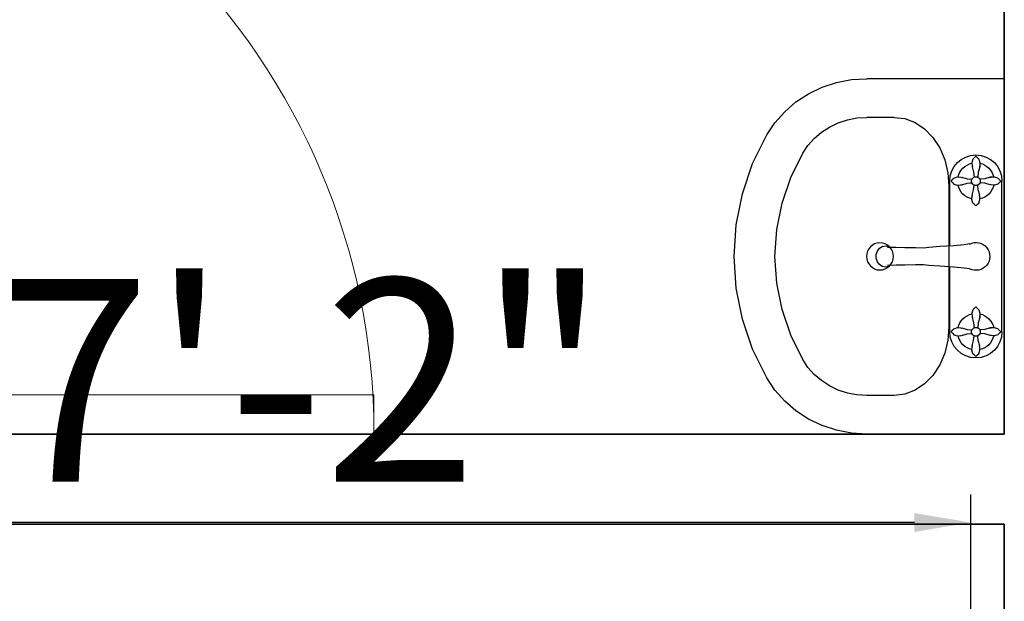
# Model space of a CAD drawing. Units: inches. Extents: x 3321 to 5237, y 11 to 1752.
# Tile 19 of 43: x 4413 to 4456, y 1280 to 1306. Entities that reach past the tile are written whole.
import ezdxf

# ---------------------------------------------------------------- set-up
doc = ezdxf.new("R2010")
doc.units = ezdxf.units.IN
for name, color, linetype, lineweight in [('A-ANNO-DIMS', 2, 'Continuous', 18), ('A-DOOR', 4, 'Continuous', 18), ('A-WALL', 7, 'Continuous', 35), ('Сантехника', 7, 'Continuous', 18)]:
    doc.layers.add(name, color=color, linetype=linetype, lineweight=lineweight)
doc.layers.add('SANTEH', color=7, linetype='Continuous')
doc.styles.get("Standard").update_dxf_attribs({"font": 'arial.ttf'})
doc.dimstyles.new('ISO-25', dxfattribs={"dimtxt": 9, "dimasz": 2.5, "dimexe": 1.25, "dimexo": 0.625, "dimtad": 1, "dimdec": 1, "dimlunit": 3, "dimtxsty": 'Standard', "dimcen": 2.5, "dimclrd": 4, "dimclre": 4, "dimclrt": 256, "dimadec": 0, "dimazin": 0, "dimtfac": 1, "dimtdec": 1, "dimtmove": 0, "dimatfit": 3, "dimfxl": 1, "dimarcsym": 0})

# ---------------------------------------------------------------- blocks, each defined once
blk = doc.blocks.new('*U5')
for p, q in [((0, 0), (0, -6)), ((-30, 0), (-30, -6))]:
    blk.add_line(p, q)
blk.add_lwpolyline([(0, 0), (0, 30), (-1.75, 30), (-1.75, 0)], close=True)
blk.add_arc((0, 0), 30, 90, 180)
blk = doc.blocks.new('Basin 01_71')
at = {"layer": 'SANTEH'}
for p, q in [((0, 350), (0, 171.8)), ((460, 350), (0, 350)), ((132.5, 345.3), (130.2, 343.2)), ((132.5, 345.3), (130.2, 343.2)), ((132.5, 345.3), (130.2, 343.2)), ((132.5, 345.3), (130.2, 343.2)), ((132.5, 345.3), (130.2, 343.2)), ((132.5, 345.3), (130.2, 343.2)), ((132.5, 346.9), (327.5, 346.9)), ((132.5, 345.3), (134.7, 343.2)), ((132.5, 345.3), (134.7, 343.2)), ((132.5, 345.3), (134.7, 343.2)), ((132.5, 345.3), (134.7, 343.2)), ((132.5, 345.3), (134.7, 343.2)), ((132.5, 345.3), (134.7, 343.2)), ((327.5, 345.3), (325.2, 343.2)), ((327.5, 345.3), (325.2, 343.2)), ((327.5, 345.3), (325.2, 343.2)), ((327.5, 345.3), (325.2, 343.2)), ((327.5, 345.3), (325.2, 343.2)), ((327.5, 345.3), (325.2, 343.2)), ((327.5, 345.3), (329.7, 343.2)), ((327.5, 345.3), (329.7, 343.2)), ((327.5, 345.3), (329.7, 343.2)), ((327.5, 345.3), (329.7, 343.2)), ((327.5, 345.3), (329.7, 343.2)), ((327.5, 345.3), (329.7, 343.2)), ((460, 350), (460, 171.8)), ((128.5, 341.7), (127.2, 337.2)), ((128.5, 341.7), (127.2, 337.2)), ((128.5, 341.7), (127.2, 337.2)), ((128.5, 341.7), (127.2, 337.2)), ((128.5, 341.7), (127.2, 337.2)), ((128.5, 341.7), (127.2, 337.2)), ((127.2, 337.2), (127.5, 332.3)), ((127.2, 337.2), (127.5, 332.3)), ((127.2, 337.2), (127.5, 332.3)), ((127.2, 337.2), (127.5, 332.3)), ((127.2, 337.2), (127.5, 332.3)), ((127.2, 337.2), (127.5, 332.3)), ((127.5, 332.3), (128.4, 332)), ((127.5, 332.3), (128.4, 332)), ((127.5, 332.3), (128.4, 332)), ((127.5, 332.3), (128.4, 332)), ((127.5, 332.3), (128.4, 332)), ((127.5, 332.3), (128.4, 332)), ((128.4, 332), (127.6, 331.5)), ((128.4, 332), (127.6, 331.5)), ((128.4, 332), (127.6, 331.5)), ((128.4, 332), (127.6, 331.5)), ((128.4, 332), (127.6, 331.5)), ((128.4, 332), (127.6, 331.5)), ((130.2, 343.2), (128.5, 341.7)), ((130.2, 343.2), (128.5, 341.7)), ((130.2, 343.2), (128.5, 341.7)), ((130.2, 343.2), (128.5, 341.7)), ((130.2, 343.2), (128.5, 341.7)), ((130.2, 343.2), (128.5, 341.7)), ((134.7, 343.2), (136.4, 341.7)), ((134.7, 343.2), (136.4, 341.7)), ((134.7, 343.2), (136.4, 341.7)), ((134.7, 343.2), (136.4, 341.7)), ((134.7, 343.2), (136.4, 341.7)), ((134.7, 343.2), (136.4, 341.7)), ((136.4, 341.7), (137.7, 337.2)), ((136.4, 341.7), (137.7, 337.2)), ((136.4, 341.7), (137.7, 337.2)), ((136.4, 341.7), (137.7, 337.2)), ((136.4, 341.7), (137.7, 337.2)), ((136.4, 341.7), (137.7, 337.2)), ((137.4, 332.3), (136.6, 332)), ((137.4, 332.3), (136.6, 332)), ((137.4, 332.3), (136.6, 332)), ((137.4, 332.3), (136.6, 332)), ((137.4, 332.3), (136.6, 332)), ((137.4, 332.3), (136.6, 332)), ((136.6, 332), (137.4, 331.5)), ((136.6, 332), (137.4, 331.5)), ((136.6, 332), (137.4, 331.5)), ((136.6, 332), (137.4, 331.5)), ((136.6, 332), (137.4, 331.5)), ((136.6, 332), (137.4, 331.5)), ((137.7, 337.2), (137.4, 332.3)), ((137.7, 337.2), (137.4, 332.3)), ((137.7, 337.2), (137.4, 332.3)), ((137.7, 337.2), (137.4, 332.3)), ((137.7, 337.2), (137.4, 332.3)), ((137.7, 337.2), (137.4, 332.3)), ((323.5, 341.7), (322.2, 337.2)), ((323.5, 341.7), (322.2, 337.2)), ((323.5, 341.7), (322.2, 337.2)), ((323.5, 341.7), (322.2, 337.2)), ((323.5, 341.7), (322.2, 337.2)), ((323.5, 341.7), (322.2, 337.2)), ((322.2, 337.2), (322.5, 332.3)), ((322.2, 337.2), (322.5, 332.3)), ((322.2, 337.2), (322.5, 332.3)), ((322.2, 337.2), (322.5, 332.3)), ((322.2, 337.2), (322.5, 332.3)), ((322.2, 337.2), (322.5, 332.3)), ((322.5, 332.3), (323.4, 332)), ((322.5, 332.3), (323.4, 332)), ((322.5, 332.3), (323.4, 332)), ((322.5, 332.3), (323.4, 332)), ((322.5, 332.3), (323.4, 332)), ((322.5, 332.3), (323.4, 332)), ((323.4, 332), (322.6, 331.5)), ((323.4, 332), (322.6, 331.5)), ((323.4, 332), (322.6, 331.5)), ((323.4, 332), (322.6, 331.5)), ((323.4, 332), (322.6, 331.5)), ((323.4, 332), (322.6, 331.5)), ((325.2, 343.2), (323.5, 341.7)), ((325.2, 343.2), (323.5, 341.7)), ((325.2, 343.2), (323.5, 341.7)), ((325.2, 343.2), (323.5, 341.7)), ((325.2, 343.2), (323.5, 341.7)), ((325.2, 343.2), (323.5, 341.7)), ((329.7, 343.2), (331.4, 341.7)), ((329.7, 343.2), (331.4, 341.7)), ((329.7, 343.2), (331.4, 341.7)), ((329.7, 343.2), (331.4, 341.7)), ((329.7, 343.2), (331.4, 341.7)), ((329.7, 343.2), (331.4, 341.7)), ((331.4, 341.7), (332.7, 337.2)), ((331.4, 341.7), (332.7, 337.2)), ((331.4, 341.7), (332.7, 337.2)), ((331.4, 341.7), (332.7, 337.2)), ((331.4, 341.7), (332.7, 337.2)), ((331.4, 341.7), (332.7, 337.2)), ((332.4, 332.3), (331.6, 332)), ((332.4, 332.3), (331.6, 332)), ((332.4, 332.3), (331.6, 332)), ((332.4, 332.3), (331.6, 332)), ((332.4, 332.3), (331.6, 332)), ((332.4, 332.3), (331.6, 332)), ((331.6, 332), (332.4, 331.5)), ((331.6, 332), (332.4, 331.5)), ((331.6, 332), (332.4, 331.5)), ((331.6, 332), (332.4, 331.5)), ((331.6, 332), (332.4, 331.5)), ((331.6, 332), (332.4, 331.5)), ((332.7, 337.2), (332.4, 332.3)), ((332.7, 337.2), (332.4, 332.3)), ((332.7, 337.2), (332.4, 332.3)), ((332.7, 337.2), (332.4, 332.3)), ((332.7, 337.2), (332.4, 332.3)), ((332.7, 337.2), (332.4, 332.3)), ((127.6, 331.5), (129.6, 324.7)), ((127.6, 331.5), (129.6, 324.7)), ((127.6, 331.5), (129.6, 324.7)), ((127.6, 331.5), (129.6, 324.7)), ((127.6, 331.5), (129.6, 324.7)), ((127.6, 331.5), (129.6, 324.7)), ((129.6, 324.7), (130.2, 318.4)), ((129.6, 324.7), (130.2, 318.4)), ((129.6, 324.7), (130.2, 318.4)), ((129.6, 324.7), (130.2, 318.4)), ((129.6, 324.7), (130.2, 318.4)), ((129.6, 324.7), (130.2, 318.4)), ((132.2, 318.9), (130.9, 318.7)), ((132.2, 318.9), (130.9, 318.7)), ((132.2, 318.9), (130.9, 318.7)), ((132.2, 318.9), (130.9, 318.7)), ((132.2, 318.9), (130.9, 318.7)), ((132.2, 318.9), (130.9, 318.7)), ((133.5, 318.8), (132.2, 318.9)), ((133.5, 318.8), (132.2, 318.9)), ((133.5, 318.8), (132.2, 318.9)), ((133.5, 318.8), (132.2, 318.9)), ((133.5, 318.8), (132.2, 318.9)), ((133.5, 318.8), (132.2, 318.9)), ((134.8, 318.4), (133.5, 318.8)), ((134.8, 318.4), (133.5, 318.8)), ((134.8, 318.4), (133.5, 318.8)), ((134.8, 318.4), (133.5, 318.8)), ((134.8, 318.4), (133.5, 318.8)), ((134.8, 318.4), (133.5, 318.8)), ((135.4, 324.7), (134.8, 318.4)), ((135.4, 324.7), (134.8, 318.4)), ((135.4, 324.7), (134.8, 318.4)), ((135.4, 324.7), (134.8, 318.4)), ((135.4, 324.7), (134.8, 318.4)), ((135.4, 324.7), (134.8, 318.4)), ((137.4, 331.5), (135.4, 324.7)), ((137.4, 331.5), (135.4, 324.7)), ((137.4, 331.5), (135.4, 324.7)), ((137.4, 331.5), (135.4, 324.7)), ((137.4, 331.5), (135.4, 324.7)), ((137.4, 331.5), (135.4, 324.7)), ((322.6, 331.5), (324.6, 324.7)), ((322.6, 331.5), (324.6, 324.7)), ((322.6, 331.5), (324.6, 324.7)), ((322.6, 331.5), (324.6, 324.7)), ((322.6, 331.5), (324.6, 324.7)), ((322.6, 331.5), (324.6, 324.7)), ((324.6, 324.7), (325.2, 318.4)), ((324.6, 324.7), (325.2, 318.4)), ((324.6, 324.7), (325.2, 318.4)), ((324.6, 324.7), (325.2, 318.4)), ((324.6, 324.7), (325.2, 318.4)), ((324.6, 324.7), (325.2, 318.4)), ((327.2, 318.9), (325.9, 318.7)), ((327.2, 318.9), (325.9, 318.7)), ((327.2, 318.9), (325.9, 318.7)), ((327.2, 318.9), (325.9, 318.7)), ((327.2, 318.9), (325.9, 318.7)), ((327.2, 318.9), (325.9, 318.7)), ((328.5, 318.8), (327.2, 318.9)), ((328.5, 318.8), (327.2, 318.9)), ((328.5, 318.8), (327.2, 318.9)), ((328.5, 318.8), (327.2, 318.9)), ((328.5, 318.8), (327.2, 318.9)), ((328.5, 318.8), (327.2, 318.9)), ((329.8, 318.4), (328.5, 318.8)), ((329.8, 318.4), (328.5, 318.8)), ((329.8, 318.4), (328.5, 318.8)), ((329.8, 318.4), (328.5, 318.8)), ((329.8, 318.4), (328.5, 318.8)), ((329.8, 318.4), (328.5, 318.8)), ((330.4, 324.7), (329.8, 318.4)), ((330.4, 324.7), (329.8, 318.4)), ((330.4, 324.7), (329.8, 318.4)), ((330.4, 324.7), (329.8, 318.4)), ((330.4, 324.7), (329.8, 318.4)), ((330.4, 324.7), (329.8, 318.4)), ((332.4, 331.5), (330.4, 324.7)), ((332.4, 331.5), (330.4, 324.7)), ((332.4, 331.5), (330.4, 324.7)), ((332.4, 331.5), (330.4, 324.7)), ((332.4, 331.5), (330.4, 324.7)), ((332.4, 331.5), (330.4, 324.7)), ((100.4, 313.2), (102.5, 315.4)), ((100.4, 313.2), (102.5, 315.4)), ((100.4, 313.2), (102.5, 315.4)), ((100.4, 313.2), (102.5, 315.4)), ((100.4, 313.2), (102.5, 315.4)), ((100.4, 313.2), (102.5, 315.4)), ((100.4, 313.2), (102.5, 310.9)), ((100.4, 313.2), (102.5, 310.9)), ((100.4, 313.2), (102.5, 310.9)), ((100.4, 313.2), (102.5, 310.9)), ((100.4, 313.2), (102.5, 310.9)), ((100.4, 313.2), (102.5, 310.9)), ((102.5, 315.4), (104, 317.1)), ((102.5, 315.4), (104, 317.1)), ((102.5, 315.4), (104, 317.1)), ((102.5, 315.4), (104, 317.1)), ((102.5, 315.4), (104, 317.1)), ((102.5, 315.4), (104, 317.1)), ((102.5, 310.9), (104, 309.2)), ((102.5, 310.9), (104, 309.2)), ((102.5, 310.9), (104, 309.2)), ((102.5, 310.9), (104, 309.2)), ((102.5, 310.9), (104, 309.2)), ((102.5, 310.9), (104, 309.2)), ((104, 317.1), (108.5, 318.4)), ((104, 317.1), (108.5, 318.4)), ((104, 317.1), (108.5, 318.4)), ((104, 317.1), (108.5, 318.4)), ((104, 317.1), (108.5, 318.4)), ((104, 317.1), (108.5, 318.4)), ((104, 309.2), (108.5, 307.9)), ((104, 309.2), (108.5, 307.9)), ((104, 309.2), (108.5, 307.9)), ((104, 309.2), (108.5, 307.9)), ((104, 309.2), (108.5, 307.9)), ((104, 309.2), (108.5, 307.9)), ((108.5, 318.4), (113.4, 318.1)), ((108.5, 318.4), (113.4, 318.1)), ((108.5, 318.4), (113.4, 318.1)), ((108.5, 318.4), (113.4, 318.1)), ((108.5, 318.4), (113.4, 318.1)), ((108.5, 318.4), (113.4, 318.1)), ((108.5, 307.9), (113.4, 308.2)), ((108.5, 307.9), (113.4, 308.2)), ((108.5, 307.9), (113.4, 308.2)), ((108.5, 307.9), (113.4, 308.2)), ((108.5, 307.9), (113.4, 308.2)), ((108.5, 307.9), (113.4, 308.2)), ((113.4, 318.1), (113.7, 317.3)), ((113.4, 318.1), (113.7, 317.3)), ((113.4, 318.1), (113.7, 317.3)), ((113.4, 318.1), (113.7, 317.3)), ((113.4, 318.1), (113.7, 317.3)), ((113.4, 318.1), (113.7, 317.3)), ((113.4, 308.2), (113.7, 309.1)), ((113.4, 308.2), (113.7, 309.1)), ((113.4, 308.2), (113.7, 309.1)), ((113.4, 308.2), (113.7, 309.1)), ((113.4, 308.2), (113.7, 309.1)), ((113.4, 308.2), (113.7, 309.1)), ((113.7, 317.3), (114.2, 318.1)), ((113.7, 317.3), (114.2, 318.1)), ((113.7, 317.3), (114.2, 318.1)), ((113.7, 317.3), (114.2, 318.1)), ((113.7, 317.3), (114.2, 318.1)), ((113.7, 317.3), (114.2, 318.1)), ((113.7, 309.1), (114.2, 308.3)), ((113.7, 309.1), (114.2, 308.3)), ((113.7, 309.1), (114.2, 308.3)), ((113.7, 309.1), (114.2, 308.3)), ((113.7, 309.1), (114.2, 308.3)), ((113.7, 309.1), (114.2, 308.3)), ((114.2, 318.1), (121, 316.1)), ((114.2, 318.1), (121, 316.1)), ((114.2, 318.1), (121, 316.1)), ((114.2, 318.1), (121, 316.1)), ((114.2, 318.1), (121, 316.1)), ((114.2, 318.1), (121, 316.1)), ((114.2, 308.3), (121, 310.3)), ((114.2, 308.3), (121, 310.3)), ((114.2, 308.3), (121, 310.3)), ((114.2, 308.3), (121, 310.3)), ((114.2, 308.3), (121, 310.3)), ((114.2, 308.3), (121, 310.3)), ((121, 316.1), (127.3, 315.5)), ((121, 316.1), (127.3, 315.5)), ((121, 316.1), (127.3, 315.5)), ((121, 316.1), (127.3, 315.5)), ((121, 316.1), (127.3, 315.5)), ((121, 316.1), (127.3, 315.5)), ((121, 310.3), (127.3, 310.9)), ((121, 310.3), (127.3, 310.9)), ((121, 310.3), (127.3, 310.9)), ((121, 310.3), (127.3, 310.9)), ((121, 310.3), (127.3, 310.9)), ((121, 310.3), (127.3, 310.9)), ((127.1, 315.1), (126.8, 313.9)), ((127.1, 315.1), (126.8, 313.9)), ((127.1, 315.1), (126.8, 313.9)), ((127.1, 315.1), (126.8, 313.9)), ((127.1, 315.1), (126.8, 313.9)), ((127.1, 315.1), (126.8, 313.9)), ((126.8, 313.9), (126.8, 312.5)), ((126.8, 313.9), (126.8, 312.5)), ((126.8, 313.9), (126.8, 312.5)), ((126.8, 313.9), (126.8, 312.5)), ((126.8, 313.9), (126.8, 312.5)), ((126.8, 313.9), (126.8, 312.5)), ((126.8, 312.5), (127.1, 311.2)), ((126.8, 312.5), (127.1, 311.2)), ((126.8, 312.5), (127.1, 311.2)), ((126.8, 312.5), (127.1, 311.2)), ((126.8, 312.5), (127.1, 311.2)), ((126.8, 312.5), (127.1, 311.2)), ((127.7, 316.3), (127.1, 315.1)), ((127.7, 316.3), (127.1, 315.1)), ((127.7, 316.3), (127.1, 315.1)), ((127.7, 316.3), (127.1, 315.1)), ((127.7, 316.3), (127.1, 315.1)), ((127.7, 316.3), (127.1, 315.1)), ((127.1, 311.2), (127.7, 310.1)), ((127.1, 311.2), (127.7, 310.1)), ((127.1, 311.2), (127.7, 310.1)), ((127.1, 311.2), (127.7, 310.1)), ((127.1, 311.2), (127.7, 310.1)), ((127.1, 311.2), (127.7, 310.1)), ((128.6, 317.3), (127.7, 316.3)), ((128.6, 317.3), (127.7, 316.3)), ((128.6, 317.3), (127.7, 316.3)), ((128.6, 317.3), (127.7, 316.3)), ((128.6, 317.3), (127.7, 316.3)), ((128.6, 317.3), (127.7, 316.3)), ((127.7, 310.1), (128.6, 309.1)), ((127.7, 310.1), (128.6, 309.1)), ((127.7, 310.1), (128.6, 309.1)), ((127.7, 310.1), (128.6, 309.1)), ((127.7, 310.1), (128.6, 309.1)), ((127.7, 310.1), (128.6, 309.1)), ((129.7, 318.1), (128.6, 317.3)), ((129.7, 318.1), (128.6, 317.3)), ((129.7, 318.1), (128.6, 317.3)), ((129.7, 318.1), (128.6, 317.3)), ((129.7, 318.1), (128.6, 317.3)), ((129.7, 318.1), (128.6, 317.3)), ((128.6, 309.1), (129.7, 308.3)), ((128.6, 309.1), (129.7, 308.3)), ((128.6, 309.1), (129.7, 308.3)), ((128.6, 309.1), (129.7, 308.3)), ((128.6, 309.1), (129.7, 308.3)), ((128.6, 309.1), (129.7, 308.3)), ((129.6, 301.7), (130.2, 308)), ((129.6, 301.7), (130.2, 308)), ((129.6, 301.7), (130.2, 308)), ((129.6, 301.7), (130.2, 308)), ((129.6, 301.7), (130.2, 308)), ((129.6, 301.7), (130.2, 308)), ((130.9, 318.7), (129.7, 318.1)), ((130.9, 318.7), (129.7, 318.1)), ((130.9, 318.7), (129.7, 318.1)), ((130.9, 318.7), (129.7, 318.1)), ((130.9, 318.7), (129.7, 318.1)), ((130.9, 318.7), (129.7, 318.1)), ((129.7, 308.3), (130.9, 307.7)), ((129.7, 308.3), (130.9, 307.7)), ((129.7, 308.3), (130.9, 307.7)), ((129.7, 308.3), (130.9, 307.7)), ((129.7, 308.3), (130.9, 307.7)), ((129.7, 308.3), (130.9, 307.7)), ((130.9, 307.7), (132.2, 307.5)), ((130.9, 307.7), (132.2, 307.5)), ((130.9, 307.7), (132.2, 307.5)), ((130.9, 307.7), (132.2, 307.5)), ((130.9, 307.7), (132.2, 307.5)), ((130.9, 307.7), (132.2, 307.5)), ((132.2, 307.5), (133.5, 307.6)), ((132.2, 307.5), (133.5, 307.6)), ((132.2, 307.5), (133.5, 307.6)), ((132.2, 307.5), (133.5, 307.6)), ((132.2, 307.5), (133.5, 307.6)), ((132.2, 307.5), (133.5, 307.6)), ((133.5, 307.6), (134.8, 308)), ((133.5, 307.6), (134.8, 308)), ((133.5, 307.6), (134.8, 308)), ((133.5, 307.6), (134.8, 308)), ((133.5, 307.6), (134.8, 308)), ((133.5, 307.6), (134.8, 308)), ((135.9, 317.8), (134.8, 318.4)), ((135.9, 317.8), (134.8, 318.4)), ((135.9, 317.8), (134.8, 318.4)), ((135.9, 317.8), (134.8, 318.4)), ((135.9, 317.8), (134.8, 318.4)), ((135.9, 317.8), (134.8, 318.4)), ((134.8, 308), (135.9, 308.6)), ((134.8, 308), (135.9, 308.6)), ((134.8, 308), (135.9, 308.6)), ((134.8, 308), (135.9, 308.6)), ((134.8, 308), (135.9, 308.6)), ((134.8, 308), (135.9, 308.6)), ((135.4, 301.7), (134.8, 308)), ((135.4, 301.7), (134.8, 308)), ((135.4, 301.7), (134.8, 308)), ((135.4, 301.7), (134.8, 308)), ((135.4, 301.7), (134.8, 308)), ((135.4, 301.7), (134.8, 308)), ((136.9, 316.9), (135.9, 317.8)), ((136.9, 316.9), (135.9, 317.8)), ((136.9, 316.9), (135.9, 317.8)), ((136.9, 316.9), (135.9, 317.8)), ((136.9, 316.9), (135.9, 317.8)), ((136.9, 316.9), (135.9, 317.8)), ((135.9, 308.6), (136.9, 309.5)), ((135.9, 308.6), (136.9, 309.5)), ((135.9, 308.6), (136.9, 309.5)), ((135.9, 308.6), (136.9, 309.5)), ((135.9, 308.6), (136.9, 309.5)), ((135.9, 308.6), (136.9, 309.5)), ((137.6, 315.8), (136.9, 316.9)), ((137.6, 315.8), (136.9, 316.9)), ((137.6, 315.8), (136.9, 316.9)), ((137.6, 315.8), (136.9, 316.9)), ((137.6, 315.8), (136.9, 316.9)), ((137.6, 315.8), (136.9, 316.9)), ((136.9, 309.5), (137.6, 310.6)), ((136.9, 309.5), (137.6, 310.6)), ((136.9, 309.5), (137.6, 310.6)), ((136.9, 309.5), (137.6, 310.6)), ((136.9, 309.5), (137.6, 310.6)), ((136.9, 309.5), (137.6, 310.6)), ((138, 314.5), (137.6, 315.8)), ((138, 314.5), (137.6, 315.8)), ((138, 314.5), (137.6, 315.8)), ((138, 314.5), (137.6, 315.8)), ((138, 314.5), (137.6, 315.8)), ((138, 314.5), (137.6, 315.8)), ((137.6, 310.6), (138, 311.9)), ((137.6, 310.6), (138, 311.9)), ((137.6, 310.6), (138, 311.9)), ((137.6, 310.6), (138, 311.9)), ((137.6, 310.6), (138, 311.9)), ((137.6, 310.6), (138, 311.9)), ((144, 316.1), (137.7, 315.5)), ((144, 316.1), (137.7, 315.5)), ((144, 316.1), (137.7, 315.5)), ((144, 316.1), (137.7, 315.5)), ((144, 316.1), (137.7, 315.5)), ((144, 316.1), (137.7, 315.5)), ((144, 310.3), (137.7, 310.9)), ((144, 310.3), (137.7, 310.9)), ((144, 310.3), (137.7, 310.9)), ((144, 310.3), (137.7, 310.9)), ((144, 310.3), (137.7, 310.9)), ((144, 310.3), (137.7, 310.9)), ((138.2, 313.2), (138, 314.5)), ((138.2, 313.2), (138, 314.5)), ((138.2, 313.2), (138, 314.5)), ((138.2, 313.2), (138, 314.5)), ((138.2, 313.2), (138, 314.5)), ((138.2, 313.2), (138, 314.5)), ((138, 311.9), (138.2, 313.2)), ((138, 311.9), (138.2, 313.2)), ((138, 311.9), (138.2, 313.2)), ((138, 311.9), (138.2, 313.2)), ((138, 311.9), (138.2, 313.2)), ((138, 311.9), (138.2, 313.2)), ((150.8, 318.1), (144, 316.1)), ((150.8, 318.1), (144, 316.1)), ((150.8, 318.1), (144, 316.1)), ((150.8, 318.1), (144, 316.1)), ((150.8, 318.1), (144, 316.1)), ((150.8, 318.1), (144, 316.1)), ((150.8, 308.3), (144, 310.3)), ((150.8, 308.3), (144, 310.3)), ((150.8, 308.3), (144, 310.3)), ((150.8, 308.3), (144, 310.3)), ((150.8, 308.3), (144, 310.3)), ((150.8, 308.3), (144, 310.3)), ((151.3, 317.3), (150.8, 318.1)), ((151.3, 317.3), (150.8, 318.1)), ((151.3, 317.3), (150.8, 318.1)), ((151.3, 317.3), (150.8, 318.1)), ((151.3, 317.3), (150.8, 318.1)), ((151.3, 317.3), (150.8, 318.1)), ((151.3, 309.1), (150.8, 308.3)), ((151.3, 309.1), (150.8, 308.3)), ((151.3, 309.1), (150.8, 308.3)), ((151.3, 309.1), (150.8, 308.3)), ((151.3, 309.1), (150.8, 308.3)), ((151.3, 309.1), (150.8, 308.3)), ((151.6, 318.1), (151.3, 317.3)), ((151.6, 318.1), (151.3, 317.3)), ((151.6, 318.1), (151.3, 317.3)), ((151.6, 318.1), (151.3, 317.3)), ((151.6, 318.1), (151.3, 317.3)), ((151.6, 318.1), (151.3, 317.3)), ((151.6, 308.3), (151.3, 309.1)), ((151.6, 308.3), (151.3, 309.1)), ((151.6, 308.3), (151.3, 309.1)), ((151.6, 308.3), (151.3, 309.1)), ((151.6, 308.3), (151.3, 309.1)), ((151.6, 308.3), (151.3, 309.1)), ((156.5, 318.4), (151.6, 318.1)), ((156.5, 318.4), (151.6, 318.1)), ((156.5, 318.4), (151.6, 318.1)), ((156.5, 318.4), (151.6, 318.1)), ((156.5, 318.4), (151.6, 318.1)), ((156.5, 318.4), (151.6, 318.1)), ((156.5, 308), (151.6, 308.3)), ((156.5, 308), (151.6, 308.3)), ((156.5, 308), (151.6, 308.3)), ((156.5, 308), (151.6, 308.3)), ((156.5, 308), (151.6, 308.3)), ((156.5, 308), (151.6, 308.3)), ((161, 317.2), (156.5, 318.4)), ((161, 317.2), (156.5, 318.4)), ((161, 317.2), (156.5, 318.4)), ((161, 317.2), (156.5, 318.4)), ((161, 317.2), (156.5, 318.4)), ((161, 317.2), (156.5, 318.4)), ((161, 309.2), (156.5, 308)), ((161, 309.2), (156.5, 308)), ((161, 309.2), (156.5, 308)), ((161, 309.2), (156.5, 308)), ((161, 309.2), (156.5, 308)), ((161, 309.2), (156.5, 308)), ((162.5, 315.4), (161, 317.2)), ((162.5, 315.4), (161, 317.2)), ((162.5, 315.4), (161, 317.2)), ((162.5, 315.4), (161, 317.2)), ((162.5, 315.4), (161, 317.2)), ((162.5, 315.4), (161, 317.2)), ((162.5, 311), (161, 309.2)), ((162.5, 311), (161, 309.2)), ((162.5, 311), (161, 309.2)), ((162.5, 311), (161, 309.2)), ((162.5, 311), (161, 309.2)), ((162.5, 311), (161, 309.2)), ((164.6, 313.2), (162.5, 315.4)), ((164.6, 313.2), (162.5, 315.4)), ((164.6, 313.2), (162.5, 315.4)), ((164.6, 313.2), (162.5, 315.4)), ((164.6, 313.2), (162.5, 315.4)), ((164.6, 313.2), (162.5, 315.4)), ((164.6, 313.2), (162.5, 311)), ((164.6, 313.2), (162.5, 311)), ((164.6, 313.2), (162.5, 311)), ((164.6, 313.2), (162.5, 311)), ((164.6, 313.2), (162.5, 311)), ((164.6, 313.2), (162.5, 311)), ((295.4, 313.2), (297.5, 315.4)), ((295.4, 313.2), (297.5, 315.4)), ((295.4, 313.2), (297.5, 315.4)), ((295.4, 313.2), (297.5, 315.4)), ((295.4, 313.2), (297.5, 315.4)), ((295.4, 313.2), (297.5, 315.4)), ((295.4, 313.2), (297.5, 310.9)), ((295.4, 313.2), (297.5, 310.9)), ((295.4, 313.2), (297.5, 310.9)), ((295.4, 313.2), (297.5, 310.9)), ((295.4, 313.2), (297.5, 310.9)), ((295.4, 313.2), (297.5, 310.9)), ((297.5, 315.4), (299, 317.1)), ((297.5, 315.4), (299, 317.1)), ((297.5, 315.4), (299, 317.1)), ((297.5, 315.4), (299, 317.1)), ((297.5, 315.4), (299, 317.1)), ((297.5, 315.4), (299, 317.1)), ((297.5, 310.9), (299, 309.2)), ((297.5, 310.9), (299, 309.2)), ((297.5, 310.9), (299, 309.2)), ((297.5, 310.9), (299, 309.2)), ((297.5, 310.9), (299, 309.2)), ((297.5, 310.9), (299, 309.2)), ((299, 317.1), (303.5, 318.4)), ((299, 317.1), (303.5, 318.4)), ((299, 317.1), (303.5, 318.4)), ((299, 317.1), (303.5, 318.4)), ((299, 317.1), (303.5, 318.4)), ((299, 317.1), (303.5, 318.4)), ((299, 309.2), (303.5, 307.9)), ((299, 309.2), (303.5, 307.9)), ((299, 309.2), (303.5, 307.9)), ((299, 309.2), (303.5, 307.9)), ((299, 309.2), (303.5, 307.9)), ((299, 309.2), (303.5, 307.9)), ((303.5, 318.4), (308.4, 318.1)), ((303.5, 318.4), (308.4, 318.1)), ((303.5, 318.4), (308.4, 318.1)), ((303.5, 318.4), (308.4, 318.1)), ((303.5, 318.4), (308.4, 318.1)), ((303.5, 318.4), (308.4, 318.1)), ((303.5, 307.9), (308.4, 308.2)), ((303.5, 307.9), (308.4, 308.2)), ((303.5, 307.9), (308.4, 308.2)), ((303.5, 307.9), (308.4, 308.2)), ((303.5, 307.9), (308.4, 308.2)), ((303.5, 307.9), (308.4, 308.2)), ((308.4, 318.1), (308.7, 317.3)), ((308.4, 318.1), (308.7, 317.3)), ((308.4, 318.1), (308.7, 317.3)), ((308.4, 318.1), (308.7, 317.3)), ((308.4, 318.1), (308.7, 317.3)), ((308.4, 318.1), (308.7, 317.3)), ((308.4, 308.2), (308.7, 309.1)), ((308.4, 308.2), (308.7, 309.1)), ((308.4, 308.2), (308.7, 309.1)), ((308.4, 308.2), (308.7, 309.1)), ((308.4, 308.2), (308.7, 309.1)), ((308.4, 308.2), (308.7, 309.1)), ((308.7, 317.3), (309.2, 318.1)), ((308.7, 317.3), (309.2, 318.1)), ((308.7, 317.3), (309.2, 318.1)), ((308.7, 317.3), (309.2, 318.1)), ((308.7, 317.3), (309.2, 318.1)), ((308.7, 317.3), (309.2, 318.1)), ((308.7, 309.1), (309.2, 308.3)), ((308.7, 309.1), (309.2, 308.3)), ((308.7, 309.1), (309.2, 308.3)), ((308.7, 309.1), (309.2, 308.3)), ((308.7, 309.1), (309.2, 308.3)), ((308.7, 309.1), (309.2, 308.3)), ((309.2, 318.1), (316, 316.1)), ((309.2, 318.1), (316, 316.1)), ((309.2, 318.1), (316, 316.1)), ((309.2, 318.1), (316, 316.1)), ((309.2, 318.1), (316, 316.1)), ((309.2, 318.1), (316, 316.1)), ((309.2, 308.3), (316, 310.3)), ((309.2, 308.3), (316, 310.3)), ((309.2, 308.3), (316, 310.3)), ((309.2, 308.3), (316, 310.3)), ((309.2, 308.3), (316, 310.3)), ((309.2, 308.3), (316, 310.3)), ((316, 316.1), (322.3, 315.5)), ((316, 316.1), (322.3, 315.5)), ((316, 316.1), (322.3, 315.5)), ((316, 316.1), (322.3, 315.5)), ((316, 316.1), (322.3, 315.5)), ((316, 316.1), (322.3, 315.5)), ((316, 310.3), (322.3, 310.9)), ((316, 310.3), (322.3, 310.9)), ((316, 310.3), (322.3, 310.9)), ((316, 310.3), (322.3, 310.9)), ((316, 310.3), (322.3, 310.9)), ((316, 310.3), (322.3, 310.9)), ((322.1, 315.1), (321.8, 313.9)), ((322.1, 315.1), (321.8, 313.9)), ((322.1, 315.1), (321.8, 313.9)), ((322.1, 315.1), (321.8, 313.9)), ((322.1, 315.1), (321.8, 313.9)), ((322.1, 315.1), (321.8, 313.9)), ((321.8, 313.9), (321.8, 312.5)), ((321.8, 313.9), (321.8, 312.5)), ((321.8, 313.9), (321.8, 312.5)), ((321.8, 313.9), (321.8, 312.5)), ((321.8, 313.9), (321.8, 312.5)), ((321.8, 313.9), (321.8, 312.5)), ((321.8, 312.5), (322.1, 311.2)), ((321.8, 312.5), (322.1, 311.2)), ((321.8, 312.5), (322.1, 311.2)), ((321.8, 312.5), (322.1, 311.2)), ((321.8, 312.5), (322.1, 311.2)), ((321.8, 312.5), (322.1, 311.2)), ((322.7, 316.3), (322.1, 315.1)), ((322.7, 316.3), (322.1, 315.1)), ((322.7, 316.3), (322.1, 315.1)), ((322.7, 316.3), (322.1, 315.1)), ((322.7, 316.3), (322.1, 315.1)), ((322.7, 316.3), (322.1, 315.1)), ((322.1, 311.2), (322.7, 310.1)), ((322.1, 311.2), (322.7, 310.1)), ((322.1, 311.2), (322.7, 310.1)), ((322.1, 311.2), (322.7, 310.1)), ((322.1, 311.2), (322.7, 310.1)), ((322.1, 311.2), (322.7, 310.1)), ((323.6, 317.3), (322.7, 316.3)), ((323.6, 317.3), (322.7, 316.3)), ((323.6, 317.3), (322.7, 316.3)), ((323.6, 317.3), (322.7, 316.3)), ((323.6, 317.3), (322.7, 316.3)), ((323.6, 317.3), (322.7, 316.3)), ((322.7, 310.1), (323.6, 309.1)), ((322.7, 310.1), (323.6, 309.1)), ((322.7, 310.1), (323.6, 309.1)), ((322.7, 310.1), (323.6, 309.1)), ((322.7, 310.1), (323.6, 309.1)), ((322.7, 310.1), (323.6, 309.1)), ((324.7, 318.1), (323.6, 317.3)), ((324.7, 318.1), (323.6, 317.3)), ((324.7, 318.1), (323.6, 317.3)), ((324.7, 318.1), (323.6, 317.3)), ((324.7, 318.1), (323.6, 317.3)), ((324.7, 318.1), (323.6, 317.3)), ((323.6, 309.1), (324.7, 308.3)), ((323.6, 309.1), (324.7, 308.3)), ((323.6, 309.1), (324.7, 308.3)), ((323.6, 309.1), (324.7, 308.3)), ((323.6, 309.1), (324.7, 308.3)), ((323.6, 309.1), (324.7, 308.3)), ((324.6, 301.7), (325.2, 308)), ((324.6, 301.7), (325.2, 308)), ((324.6, 301.7), (325.2, 308)), ((324.6, 301.7), (325.2, 308)), ((324.6, 301.7), (325.2, 308)), ((324.6, 301.7), (325.2, 308)), ((325.9, 318.7), (324.7, 318.1)), ((325.9, 318.7), (324.7, 318.1)), ((325.9, 318.7), (324.7, 318.1)), ((325.9, 318.7), (324.7, 318.1)), ((325.9, 318.7), (324.7, 318.1)), ((325.9, 318.7), (324.7, 318.1)), ((324.7, 308.3), (325.9, 307.7)), ((324.7, 308.3), (325.9, 307.7)), ((324.7, 308.3), (325.9, 307.7)), ((324.7, 308.3), (325.9, 307.7)), ((324.7, 308.3), (325.9, 307.7)), ((324.7, 308.3), (325.9, 307.7)), ((325.9, 307.7), (327.2, 307.5)), ((325.9, 307.7), (327.2, 307.5)), ((325.9, 307.7), (327.2, 307.5)), ((325.9, 307.7), (327.2, 307.5)), ((325.9, 307.7), (327.2, 307.5)), ((325.9, 307.7), (327.2, 307.5)), ((327.2, 307.5), (328.5, 307.6)), ((327.2, 307.5), (328.5, 307.6)), ((327.2, 307.5), (328.5, 307.6)), ((327.2, 307.5), (328.5, 307.6)), ((327.2, 307.5), (328.5, 307.6)), ((327.2, 307.5), (328.5, 307.6)), ((328.5, 307.6), (329.8, 308)), ((328.5, 307.6), (329.8, 308)), ((328.5, 307.6), (329.8, 308)), ((328.5, 307.6), (329.8, 308)), ((328.5, 307.6), (329.8, 308)), ((328.5, 307.6), (329.8, 308)), ((330.9, 317.8), (329.8, 318.4)), ((330.9, 317.8), (329.8, 318.4)), ((330.9, 317.8), (329.8, 318.4)), ((330.9, 317.8), (329.8, 318.4)), ((330.9, 317.8), (329.8, 318.4)), ((330.9, 317.8), (329.8, 318.4)), ((329.8, 308), (330.9, 308.6)), ((329.8, 308), (330.9, 308.6)), ((329.8, 308), (330.9, 308.6)), ((329.8, 308), (330.9, 308.6)), ((329.8, 308), (330.9, 308.6)), ((329.8, 308), (330.9, 308.6)), ((330.4, 301.7), (329.8, 308)), ((330.4, 301.7), (329.8, 308)), ((330.4, 301.7), (329.8, 308)), ((330.4, 301.7), (329.8, 308)), ((330.4, 301.7), (329.8, 308)), ((330.4, 301.7), (329.8, 308)), ((331.9, 316.9), (330.9, 317.8)), ((331.9, 316.9), (330.9, 317.8)), ((331.9, 316.9), (330.9, 317.8)), ((331.9, 316.9), (330.9, 317.8)), ((331.9, 316.9), (330.9, 317.8)), ((331.9, 316.9), (330.9, 317.8)), ((330.9, 308.6), (331.9, 309.5)), ((330.9, 308.6), (331.9, 309.5)), ((330.9, 308.6), (331.9, 309.5)), ((330.9, 308.6), (331.9, 309.5)), ((330.9, 308.6), (331.9, 309.5)), ((330.9, 308.6), (331.9, 309.5)), ((332.6, 315.8), (331.9, 316.9)), ((332.6, 315.8), (331.9, 316.9)), ((332.6, 315.8), (331.9, 316.9)), ((332.6, 315.8), (331.9, 316.9)), ((332.6, 315.8), (331.9, 316.9)), ((332.6, 315.8), (331.9, 316.9)), ((331.9, 309.5), (332.6, 310.6)), ((331.9, 309.5), (332.6, 310.6)), ((331.9, 309.5), (332.6, 310.6)), ((331.9, 309.5), (332.6, 310.6)), ((331.9, 309.5), (332.6, 310.6)), ((331.9, 309.5), (332.6, 310.6)), ((333, 314.5), (332.6, 315.8)), ((333, 314.5), (332.6, 315.8)), ((333, 314.5), (332.6, 315.8)), ((333, 314.5), (332.6, 315.8)), ((333, 314.5), (332.6, 315.8)), ((333, 314.5), (332.6, 315.8)), ((332.6, 310.6), (333, 311.9)), ((332.6, 310.6), (333, 311.9)), ((332.6, 310.6), (333, 311.9)), ((332.6, 310.6), (333, 311.9)), ((332.6, 310.6), (333, 311.9)), ((332.6, 310.6), (333, 311.9)), ((339, 316.1), (332.7, 315.5)), ((339, 316.1), (332.7, 315.5)), ((339, 316.1), (332.7, 315.5)), ((339, 316.1), (332.7, 315.5)), ((339, 316.1), (332.7, 315.5)), ((339, 316.1), (332.7, 315.5)), ((339, 310.3), (332.7, 310.9)), ((339, 310.3), (332.7, 310.9)), ((339, 310.3), (332.7, 310.9)), ((339, 310.3), (332.7, 310.9)), ((339, 310.3), (332.7, 310.9)), ((339, 310.3), (332.7, 310.9)), ((333.2, 313.2), (333, 314.5)), ((333.2, 313.2), (333, 314.5)), ((333.2, 313.2), (333, 314.5)), ((333.2, 313.2), (333, 314.5)), ((333.2, 313.2), (333, 314.5)), ((333.2, 313.2), (333, 314.5)), ((333, 311.9), (333.2, 313.2)), ((333, 311.9), (333.2, 313.2)), ((333, 311.9), (333.2, 313.2)), ((333, 311.9), (333.2, 313.2)), ((333, 311.9), (333.2, 313.2)), ((333, 311.9), (333.2, 313.2)), ((345.8, 318.1), (339, 316.1)), ((345.8, 318.1), (339, 316.1)), ((345.8, 318.1), (339, 316.1)), ((345.8, 318.1), (339, 316.1)), ((345.8, 318.1), (339, 316.1)), ((345.8, 318.1), (339, 316.1)), ((345.8, 308.3), (339, 310.3)), ((345.8, 308.3), (339, 310.3)), ((345.8, 308.3), (339, 310.3)), ((345.8, 308.3), (339, 310.3)), ((345.8, 308.3), (339, 310.3)), ((345.8, 308.3), (339, 310.3)), ((346.3, 317.3), (345.8, 318.1)), ((346.3, 317.3), (345.8, 318.1)), ((346.3, 317.3), (345.8, 318.1)), ((346.3, 317.3), (345.8, 318.1)), ((346.3, 317.3), (345.8, 318.1)), ((346.3, 317.3), (345.8, 318.1)), ((346.3, 309.1), (345.8, 308.3)), ((346.3, 309.1), (345.8, 308.3)), ((346.3, 309.1), (345.8, 308.3)), ((346.3, 309.1), (345.8, 308.3)), ((346.3, 309.1), (345.8, 308.3)), ((346.3, 309.1), (345.8, 308.3)), ((346.6, 318.1), (346.3, 317.3)), ((346.6, 318.1), (346.3, 317.3)), ((346.6, 318.1), (346.3, 317.3)), ((346.6, 318.1), (346.3, 317.3)), ((346.6, 318.1), (346.3, 317.3)), ((346.6, 318.1), (346.3, 317.3)), ((346.6, 308.3), (346.3, 309.1)), ((346.6, 308.3), (346.3, 309.1)), ((346.6, 308.3), (346.3, 309.1)), ((346.6, 308.3), (346.3, 309.1)), ((346.6, 308.3), (346.3, 309.1)), ((346.6, 308.3), (346.3, 309.1)), ((351.5, 318.4), (346.6, 318.1)), ((351.5, 318.4), (346.6, 318.1)), ((351.5, 318.4), (346.6, 318.1)), ((351.5, 318.4), (346.6, 318.1)), ((351.5, 318.4), (346.6, 318.1)), ((351.5, 318.4), (346.6, 318.1)), ((351.5, 308), (346.6, 308.3)), ((351.5, 308), (346.6, 308.3)), ((351.5, 308), (346.6, 308.3)), ((351.5, 308), (346.6, 308.3)), ((351.5, 308), (346.6, 308.3)), ((351.5, 308), (346.6, 308.3)), ((356, 317.2), (351.5, 318.4)), ((356, 317.2), (351.5, 318.4)), ((356, 317.2), (351.5, 318.4)), ((356, 317.2), (351.5, 318.4)), ((356, 317.2), (351.5, 318.4)), ((356, 317.2), (351.5, 318.4)), ((356, 309.2), (351.5, 308)), ((356, 309.2), (351.5, 308)), ((356, 309.2), (351.5, 308)), ((356, 309.2), (351.5, 308)), ((356, 309.2), (351.5, 308)), ((356, 309.2), (351.5, 308)), ((357.5, 315.4), (356, 317.2)), ((357.5, 315.4), (356, 317.2)), ((357.5, 315.4), (356, 317.2)), ((357.5, 315.4), (356, 317.2)), ((357.5, 315.4), (356, 317.2)), ((357.5, 315.4), (356, 317.2)), ((357.5, 311), (356, 309.2)), ((357.5, 311), (356, 309.2)), ((357.5, 311), (356, 309.2)), ((357.5, 311), (356, 309.2)), ((357.5, 311), (356, 309.2)), ((357.5, 311), (356, 309.2)), ((359.6, 313.2), (357.5, 315.4)), ((359.6, 313.2), (357.5, 315.4)), ((359.6, 313.2), (357.5, 315.4)), ((359.6, 313.2), (357.5, 315.4)), ((359.6, 313.2), (357.5, 315.4)), ((359.6, 313.2), (357.5, 315.4)), ((359.6, 313.2), (357.5, 311)), ((359.6, 313.2), (357.5, 311)), ((359.6, 313.2), (357.5, 311)), ((359.6, 313.2), (357.5, 311)), ((359.6, 313.2), (357.5, 311)), ((359.6, 313.2), (357.5, 311)), ((127.3, 289.2), (127.6, 294.1)), ((127.3, 289.2), (127.6, 294.1)), ((127.3, 289.2), (127.6, 294.1)), ((127.3, 289.2), (127.6, 294.1)), ((127.3, 289.2), (127.6, 294.1)), ((127.3, 289.2), (127.6, 294.1)), ((127.6, 294.9), (129.6, 301.7)), ((127.6, 294.9), (129.6, 301.7)), ((127.6, 294.9), (129.6, 301.7)), ((127.6, 294.9), (129.6, 301.7)), ((127.6, 294.9), (129.6, 301.7)), ((127.6, 294.9), (129.6, 301.7)), ((128.4, 294.4), (127.6, 294.9)), ((128.4, 294.4), (127.6, 294.9)), ((128.4, 294.4), (127.6, 294.9)), ((128.4, 294.4), (127.6, 294.9)), ((128.4, 294.4), (127.6, 294.9)), ((128.4, 294.4), (127.6, 294.9)), ((127.6, 294.1), (128.4, 294.4)), ((127.6, 294.1), (128.4, 294.4)), ((127.6, 294.1), (128.4, 294.4)), ((127.6, 294.1), (128.4, 294.4)), ((127.6, 294.1), (128.4, 294.4)), ((127.6, 294.1), (128.4, 294.4)), ((137.4, 294.9), (135.4, 301.7)), ((137.4, 294.9), (135.4, 301.7)), ((137.4, 294.9), (135.4, 301.7)), ((137.4, 294.9), (135.4, 301.7)), ((137.4, 294.9), (135.4, 301.7)), ((137.4, 294.9), (135.4, 301.7)), ((136.6, 294.4), (137.4, 294.9)), ((136.6, 294.4), (137.4, 294.9)), ((136.6, 294.4), (137.4, 294.9)), ((136.6, 294.4), (137.4, 294.9)), ((136.6, 294.4), (137.4, 294.9)), ((136.6, 294.4), (137.4, 294.9)), ((137.5, 294.1), (136.6, 294.4)), ((137.5, 294.1), (136.6, 294.4)), ((137.5, 294.1), (136.6, 294.4)), ((137.5, 294.1), (136.6, 294.4)), ((137.5, 294.1), (136.6, 294.4)), ((137.5, 294.1), (136.6, 294.4)), ((137.8, 289.2), (137.5, 294.1)), ((137.8, 289.2), (137.5, 294.1)), ((137.8, 289.2), (137.5, 294.1)), ((137.8, 289.2), (137.5, 294.1)), ((137.8, 289.2), (137.5, 294.1)), ((137.8, 289.2), (137.5, 294.1)), ((213.9, 305.1), (215, 298)), ((215, 298), (216.2, 284.6)), ((245, 298), (243.8, 284.6)), ((246.1, 305.1), (245, 298)), ((322.3, 289.2), (322.6, 294.1)), ((322.3, 289.2), (322.6, 294.1)), ((322.3, 289.2), (322.6, 294.1)), ((322.3, 289.2), (322.6, 294.1)), ((322.3, 289.2), (322.6, 294.1)), ((322.3, 289.2), (322.6, 294.1)), ((322.6, 294.9), (324.6, 301.7)), ((322.6, 294.9), (324.6, 301.7)), ((322.6, 294.9), (324.6, 301.7)), ((322.6, 294.9), (324.6, 301.7)), ((322.6, 294.9), (324.6, 301.7)), ((322.6, 294.9), (324.6, 301.7)), ((323.4, 294.4), (322.6, 294.9)), ((323.4, 294.4), (322.6, 294.9)), ((323.4, 294.4), (322.6, 294.9)), ((323.4, 294.4), (322.6, 294.9)), ((323.4, 294.4), (322.6, 294.9)), ((323.4, 294.4), (322.6, 294.9)), ((322.6, 294.1), (323.4, 294.4)), ((322.6, 294.1), (323.4, 294.4)), ((322.6, 294.1), (323.4, 294.4)), ((322.6, 294.1), (323.4, 294.4)), ((322.6, 294.1), (323.4, 294.4)), ((322.6, 294.1), (323.4, 294.4)), ((332.4, 294.9), (330.4, 301.7)), ((332.4, 294.9), (330.4, 301.7)), ((332.4, 294.9), (330.4, 301.7)), ((332.4, 294.9), (330.4, 301.7)), ((332.4, 294.9), (330.4, 301.7)), ((332.4, 294.9), (330.4, 301.7)), ((331.6, 294.4), (332.4, 294.9)), ((331.6, 294.4), (332.4, 294.9)), ((331.6, 294.4), (332.4, 294.9)), ((331.6, 294.4), (332.4, 294.9)), ((331.6, 294.4), (332.4, 294.9)), ((331.6, 294.4), (332.4, 294.9)), ((332.5, 294.1), (331.6, 294.4)), ((332.5, 294.1), (331.6, 294.4)), ((332.5, 294.1), (331.6, 294.4)), ((332.5, 294.1), (331.6, 294.4)), ((332.5, 294.1), (331.6, 294.4)), ((332.5, 294.1), (331.6, 294.4)), ((332.8, 289.2), (332.5, 294.1)), ((332.8, 289.2), (332.5, 294.1)), ((332.8, 289.2), (332.5, 294.1)), ((332.8, 289.2), (332.5, 294.1)), ((332.8, 289.2), (332.5, 294.1)), ((332.8, 289.2), (332.5, 294.1)), ((128.6, 284.7), (127.3, 289.2)), ((128.6, 284.7), (127.3, 289.2)), ((128.6, 284.7), (127.3, 289.2)), ((128.6, 284.7), (127.3, 289.2)), ((128.6, 284.7), (127.3, 289.2)), ((128.6, 284.7), (127.3, 289.2)), ((130.3, 283.2), (128.6, 284.7)), ((130.3, 283.2), (128.6, 284.7)), ((130.3, 283.2), (128.6, 284.7)), ((130.3, 283.2), (128.6, 284.7)), ((130.3, 283.2), (128.6, 284.7)), ((130.3, 283.2), (128.6, 284.7)), ((132.5, 281.1), (130.3, 283.2)), ((132.5, 281.1), (130.3, 283.2)), ((132.5, 281.1), (130.3, 283.2)), ((132.5, 281.1), (130.3, 283.2)), ((132.5, 281.1), (130.3, 283.2)), ((132.5, 281.1), (130.3, 283.2)), ((132.5, 281.1), (134.8, 283.2)), ((132.5, 281.1), (134.8, 283.2)), ((132.5, 281.1), (134.8, 283.2)), ((132.5, 281.1), (134.8, 283.2)), ((132.5, 281.1), (134.8, 283.2)), ((132.5, 281.1), (134.8, 283.2)), ((134.8, 283.2), (136.5, 284.7)), ((134.8, 283.2), (136.5, 284.7)), ((134.8, 283.2), (136.5, 284.7)), ((134.8, 283.2), (136.5, 284.7)), ((134.8, 283.2), (136.5, 284.7)), ((134.8, 283.2), (136.5, 284.7)), ((136.5, 284.7), (137.8, 289.2)), ((136.5, 284.7), (137.8, 289.2)), ((136.5, 284.7), (137.8, 289.2)), ((136.5, 284.7), (137.8, 289.2)), ((136.5, 284.7), (137.8, 289.2)), ((136.5, 284.7), (137.8, 289.2)), ((216.2, 284.6), (217.3, 266.6)), ((243.8, 284.6), (242.7, 266.6)), ((323.6, 284.7), (322.3, 289.2)), ((323.6, 284.7), (322.3, 289.2)), ((323.6, 284.7), (322.3, 289.2)), ((323.6, 284.7), (322.3, 289.2)), ((323.6, 284.7), (322.3, 289.2)), ((323.6, 284.7), (322.3, 289.2)), ((325.3, 283.2), (323.6, 284.7)), ((325.3, 283.2), (323.6, 284.7)), ((325.3, 283.2), (323.6, 284.7)), ((325.3, 283.2), (323.6, 284.7)), ((325.3, 283.2), (323.6, 284.7)), ((325.3, 283.2), (323.6, 284.7)), ((327.5, 281.1), (325.3, 283.2)), ((327.5, 281.1), (325.3, 283.2)), ((327.5, 281.1), (325.3, 283.2)), ((327.5, 281.1), (325.3, 283.2)), ((327.5, 281.1), (325.3, 283.2)), ((327.5, 281.1), (325.3, 283.2)), ((327.5, 281.1), (329.8, 283.2)), ((327.5, 281.1), (329.8, 283.2)), ((327.5, 281.1), (329.8, 283.2)), ((327.5, 281.1), (329.8, 283.2)), ((327.5, 281.1), (329.8, 283.2)), ((327.5, 281.1), (329.8, 283.2)), ((329.8, 283.2), (331.5, 284.7)), ((329.8, 283.2), (331.5, 284.7)), ((329.8, 283.2), (331.5, 284.7)), ((329.8, 283.2), (331.5, 284.7)), ((329.8, 283.2), (331.5, 284.7)), ((329.8, 283.2), (331.5, 284.7)), ((331.5, 284.7), (332.8, 289.2)), ((331.5, 284.7), (332.8, 289.2)), ((331.5, 284.7), (332.8, 289.2)), ((331.5, 284.7), (332.8, 289.2)), ((331.5, 284.7), (332.8, 289.2)), ((331.5, 284.7), (332.8, 289.2)), ((132.5, 279.4), (216.5, 279.4)), ((138.9, 278.2), (138.9, 278.2)), ((321.1, 278.2), (138.9, 278.2)), ((243.5, 279.4), (327.5, 279.4)), ((217.3, 266.6), (218.3, 252.4)), ((242.7, 266.6), (241.7, 252.4)), ((218.3, 252.4), (219.3, 245.4)), ((219.3, 245.4), (219, 234.8)), ((241.7, 252.4), (240.7, 245.4)), ((240.7, 245.4), (241, 234.8)), ((219, 234.8), (218.8, 221.1)), ((241, 234.8), (241.2, 221.1)), ((218.8, 221.1), (218.6, 209.8)), ((241.2, 221.1), (241.4, 209.8)), ((50, 207.5), (50, 171.8)), ((218.6, 209.8), (218.4, 198.7)), ((241.4, 209.8), (241.6, 198.7)), ((410, 207.5), (410, 171.8)), ((217, 200.3), (216.2, 196.2)), ((216.2, 196.2), (217, 192.1)), ((217.1, 200.6), (217, 200.3)), ((217, 192.1), (217.1, 191.8)), ((218.5, 202.5), (217.1, 200.6)), ((217.1, 191.8), (219.5, 188.3)), ((240.5, 188.3), (242.9, 191.8)), ((242.9, 200.6), (241.5, 202.5)), ((242.9, 200.6), (243, 200.3)), ((243, 192.1), (242.9, 191.8)), ((243.8, 196.2), (243, 200.3)), ((243, 192.1), (243.8, 196.2)), ((219.5, 188.3), (223.2, 185.6)), ((223.2, 185.6), (227.6, 184.2)), ((227.6, 184.2), (227.7, 184.2)), ((227.7, 184.2), (232.3, 184.2)), ((232.4, 184.2), (232.3, 184.2)), ((232.4, 184.2), (236.8, 185.6)), ((236.8, 185.6), (240.5, 188.3))]:
    blk.add_line(p, q, dxfattribs=at)
for points in [[(138.9, 278.2), (121.6, 276.9), (104.9, 272.8), (89.5, 266.3), (76, 257.5), (65, 246.8), (56.8, 234.5), (51.7, 221.3), (50, 207.5)], [(410, 207.5), (408.3, 221.3), (403.2, 234.5), (395, 246.8), (384, 257.5), (370.5, 266.3), (355.1, 272.8), (338.4, 276.9), (321.1, 278.2)], [(0, 171.8), (1.2, 152.1), (5, 132.7), (11.1, 114.1), (19.5, 96.5), (30.1, 80.2), (42.7, 65.6), (56.9, 52.9), (72.7, 42.3)], [(50, 171.8), (50.8, 159.2), (53.2, 146.8), (57.1, 134.9), (62.5, 123.6), (69.3, 113.2), (77.3, 103.8), (86.4, 95.7), (96.5, 89)], [(363.5, 89), (373.6, 95.7), (382.7, 103.8), (390.7, 113.2), (397.5, 123.6), (402.9, 134.9), (406.8, 146.8), (409.2, 159.2), (410, 171.8)], [(387.3, 42.3), (403.1, 52.9), (417.3, 65.6), (429.9, 80.2), (440.5, 96.5), (448.9, 114.1), (455, 132.7), (458.8, 152.1), (460, 171.8)], [(96.5, 89), (128, 73.4), (161.1, 62.2), (195.3, 55.3), (230, 53), (264.7, 55.3), (298.9, 62.2), (332, 73.4), (363.5, 89)], [(72.7, 42.3), (109.8, 24), (148.8, 10.8), (189.1, 2.7), (230, 0), (270.9, 2.7), (311.2, 10.8), (350.2, 24), (387.3, 42.3)]]:
    blk.add_lwpolyline(points, dxfattribs=at)
blk.add_circle((230, 188.9), 17.5, dxfattribs=at)
for centre, radius, start, end in [((132.5, 313.2), 33.8, 90, 270), ((327.5, 313.2), 33.8, 270, 90), ((132.5, 313.2), 23.7, 102.6646, 167.4213), ((132.5, 313.2), 23.7, 12.6646, 77.4213), ((327.5, 313.2), 23.7, 102.5787, 167.3354), ((327.5, 313.2), 23.7, 12.5787, 77.3354), ((230, 313.2), 18, 333.1469, 206.8531), ((132.5, 313.2), 23.7, 192.6646, 257.4213), ((132.5, 313.2), 23.7, 282.6646, 347.4213), ((327.5, 313.2), 23.7, 192.5787, 257.3354), ((327.5, 313.2), 23.7, 282.5787, 347.3354)]:
    blk.add_arc(centre, radius, start, end, dxfattribs=at)
blk = doc.blocks.new('*D195')
at = {"layer": 'A-ANNO-DIMS', "color": 4, "lineweight": -2, "transparency": 16777216}
for p, q in [((4369.073, 1271.165), (4369.073, 1284.663)), ((4454.896, 1271.165), (4454.896, 1284.663)), ((4452.396, 1283.413), (4371.573, 1283.413))]:
    blk.add_line(p, q, dxfattribs=at)
at = {"layer": 'A-ANNO-DIMS', "color": 4, "transparency": 16777216}
for points in [[(4371.573, 1283.83), (4371.573, 1282.997), (4369.073, 1283.413)], [(4452.396, 1283.83), (4452.396, 1282.997), (4454.896, 1283.413)]]:
    blk.add_solid(points, dxfattribs=at)
at = {"layer": 'Defpoints', "color": 0, "transparency": 16777216}
for p in [(4369.073, 1283.413), (4369.073, 1270.54), (4454.896, 1270.54)]:
    blk.add_point(p, dxfattribs=at)
at = {"layer": 'A-ANNO-DIMS', "transparency": 16777216, "insert": (4411.984, 1288.56), "char_height": 9, "attachment_point": 5}
blk.add_mtext('BED 7\'-2"', dxfattribs=at)

msp = doc.modelspace()

# ---------------------------------------------------------------- linework, layer by layer
at = {"layer": 'A-WALL'}
for p, q in [((4456.386, 1371.339), (4456.386, 1287.339)), ((4376.386, 1287.339), (4456.386, 1287.339)), ((4376.386, 1283.339), (4456.386, 1283.339)), ((4456.386, 1283.339), (4456.386, 1181.339))]:
    msp.add_line(p, q, dxfattribs=at)

# ---------------------------------------------------------------- block references
at = {"layer": 'A-DOOR', "rotation": 270}
msp.add_blockref('*U5', (4398.386, 1287.339), dxfattribs=at)
at = {"layer": 'Сантехника', "xscale": -0.0343047947041041, "yscale": 0.0343047947041041, "zscale": 0.0343047947041041, "rotation": 270}
msp.add_blockref('Basin 01_71', (4444.38, 1287.338), dxfattribs=at)

# ---------------------------------------------------------------- dimensions: what is measured, and where the dimension line sits
at = {"layer": 'A-ANNO-DIMS'}
dim = msp.add_linear_dim(base=(4369.073, 1283.413), p1=(4454.896, 1270.54), p2=(4369.073, 1270.54), angle=180, text='BED <>', dimstyle='ISO-25', override={"dimdec": 1, "dimlfac": 1, "dimrnd": 0, "dimzin": 1, "dimdsep": 46, "dimlunit": 4, "dimfrac": 2}, dxfattribs=at)
dim.commit()
dim.dimension.update_dxf_attribs({"geometry": '*D195', "text_midpoint": (4411.984, 1288.56)})

doc.saveas('drawing.dxf')
